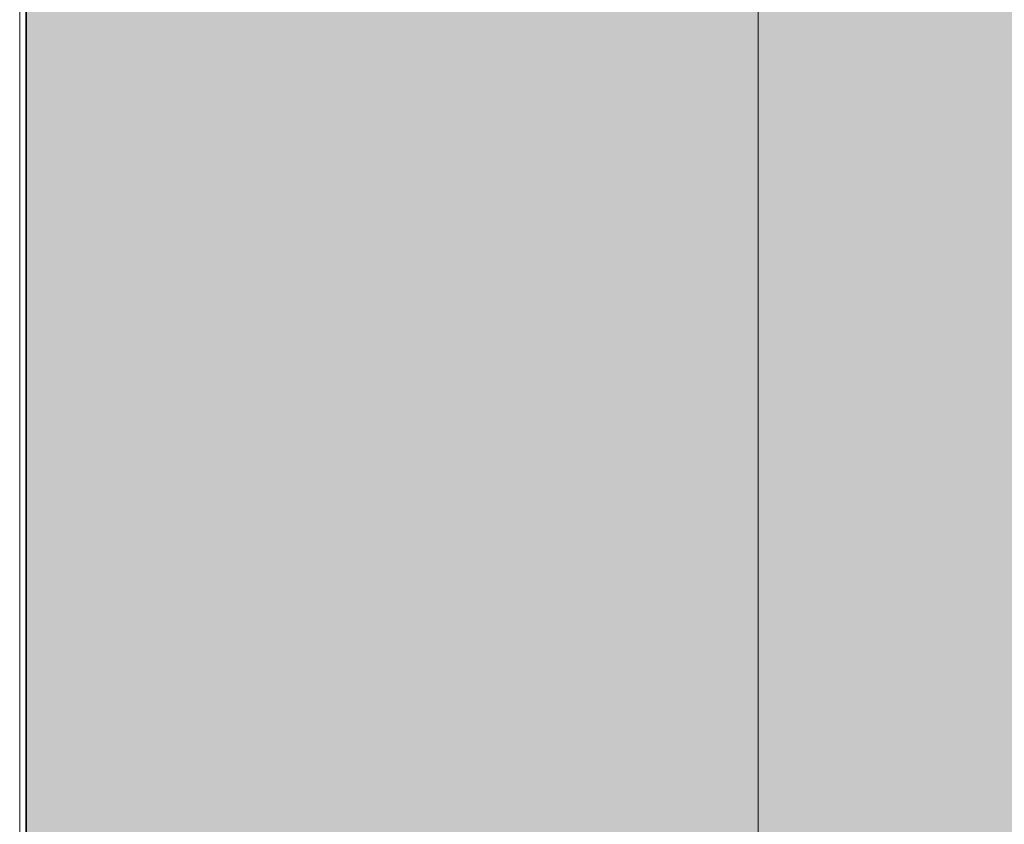
# Model space of a CAD drawing. Units: inches. Extents: x 2091 to 2899, y 967 to 2217.
# Tile 237 of 256: x 2203.116 to 2207.329, y 1155.69 to 1159.133. Entities that reach past the tile are written whole.
import ezdxf

# ---------------------------------------------------------------- set-up
doc = ezdxf.new("R2010")
doc.units = ezdxf.units.IN
doc.layers.add('A-GLAZ', color=4, linetype='Continuous', lineweight=18)
doc.layers.add('C-PROP', color=7, linetype='Continuous', lineweight=35)
doc.layers.add('A-WALL-PATT', color=141, linetype='Continuous', lineweight=13, true_color=0xadddf7)

# ---------------------------------------------------------------- blocks, each defined once
blk = doc.blocks.new('WIN-DOUBLE-LINE')
for p, q in [((0.0004, -0.0004), (0.0004, 80.8229)), ((3.1603, 80.8229), (3.1603, -0.0004))]:
    blk.add_line(p, q)

msp = doc.modelspace()

# ---------------------------------------------------------------- hatches: boundary and pattern name
at = {"layer": 'A-WALL-PATT'}
h = msp.add_hatch(color=256, dxfattribs=at)
h.dxf.hatch_style = 1
h.paths.add_polyline_path([(2803.1436, 2050.9191), (2203.1436, 2050.9191), (2203.1436, 1090.9191), (2803.1436, 1090.9191)])
h.paths.add_polyline_path([(2635.7989, 1147.5405), (2674.5241, 1147.5405, 0.376086), (2678.5297, 1152.8802), (2678.5297, 1159.5565, 0.333335), (2674.5243, 1163.5618), (2674.5243, 1163.5619), (2674.5243, 1192.9344), (2635.806, 1192.9344), (2597.0876, 1192.9344), (2597.0876, 1163.5618, 0.333335), (2593.0823, 1159.5565), (2593.0823, 1152.8802, 0.376086), (2597.0879, 1147.5405)], flags=0)
h.paths.add_polyline_path([(2436.0104, 1278.2408, 0.000483), (2435.9526, 1278.215, -0.001328), (2435.9356, 1278.1117, -0.001711), (2436.1164, 1278.0408, 0.002185)], flags=0)
h.paths.add_polyline_path([(2794.1436, 1143.4191), (2794.1436, 1347.4191), (2543.3702, 1347.4191), (2543.3702, 1351.9191), (2794.1436, 1351.9191), (2794.1436, 1392.7136), (2793.9474, 1392.7136), (2793.9474, 1473.5369), (2794.1436, 1473.5369), (2794.1436, 1531.9191), (2650.1436, 1531.9191), (2650.1436, 1536.4191), (2794.1436, 1536.4191), (2794.1436, 1692.4191), (2609.3756, 1692.4191), (2609.3756, 1644.4191), (2604.8756, 1644.4191), (2604.8756, 1744.9191), (2609.3756, 1744.9191), (2609.3756, 1696.9191), (2794.1436, 1696.9191), (2794.1436, 1780.9191), (2609.6436, 1780.9191), (2493.8756, 1780.9191), (2493.8756, 1785.4191), (2609.6436, 1785.4191), (2794.1436, 1785.4191), (2794.1436, 1847.9388), (2793.9512, 1847.9388), (2793.9512, 1928.7622), (2794.1436, 1928.7622), (2794.1436, 1941.4191), (2614.1436, 1941.4191), (2614.1436, 1821.4191), (2609.6436, 1821.4191), (2609.6436, 1941.4191), (2392.1436, 1941.4191), (2392.1436, 1819.9191), (2387.6436, 1819.9191), (2387.6436, 1941.4191), (2212.1436, 1941.4191), (2212.1436, 1783.9191), (2392.1436, 1783.9191), (2392.1436, 1780.9191), (2212.1436, 1780.9191), (2212.1436, 1629.4191), (2387.6436, 1629.4191), (2387.6436, 1744.9191), (2392.1436, 1744.9191), (2392.1436, 1627.9191), (2317.1436, 1627.9191), (2317.1436, 1551.4191), (2317.1436, 1536.4191), (2459.3836, 1536.4191), (2459.3836, 1602.3965), (2463.8836, 1602.3965), (2463.8836, 1531.9191), (2456.6436, 1531.9191), (2456.6436, 1529.9191), (2452.1436, 1529.9191), (2452.1436, 1531.9191), (2312.6436, 1531.9191), (2312.6436, 1551.4191), (2306.1436, 1551.4191), (2306.1436, 1555.9191), (2308.1436, 1555.9191), (2308.1436, 1551.4191), (2312.6436, 1551.4191), (2312.6436, 1627.9191), (2212.1436, 1627.9191), (2212.1436, 1555.9191), (2270.1436, 1555.9191), (2270.1436, 1551.4191), (2212.1436, 1551.4191), (2212.1436, 1351.9191), (2272.1436, 1351.9191), (2272.1436, 1347.4191), (2212.1436, 1347.4191), (2212.1436, 1275.4191), (2308.1436, 1275.4191), (2308.1436, 1351.9191), (2452.1436, 1351.9191), (2452.1436, 1493.9191), (2456.6436, 1493.9191), (2456.6436, 1347.4191), (2312.6436, 1347.4191), (2312.6436, 1270.9191), (2212.1436, 1270.9191), (2212.1436, 1099.9191), (2281.2375, 1099.9191), (2282.871, 1110.9138), (2282.0083, 1116.9966), (2278.5577, 1121.4204), (2268.2056, 1128.0562), (2272.0876, 1128.0562), (2273.8129, 1131.927), (2279.4203, 1134.6919), (2285.0278, 1135.2449), (2287.6158, 1137.4568), (2288.0471, 1138.0098), (2289.3411, 1140.7747), (2291.0665, 1139.6687), (2292.3605, 1135.2449), (2295.3798, 1136.9038), (2296.2425, 1135.7979), (2297.1052, 1133.033), (2300.1246, 1138.0098), (2303.1439, 1138.0098), (2304.4379, 1135.7979), (2303.1439, 1133.586), (2306.5946, 1134.6919), (2307.8887, 1133.033), (2310.908, 1135.2449), (2313.9274, 1134.1389), (2315.6269, 1132.4271), (2308.32, 1117.5496), (2290.2038, 1109.8079), (2288.9098, 1103.1721), (2289.2723, 1099.9191), (2434.9182, 1099.9191), (2431.5932, 1124.7881), (2429.9302, 1169.5531), (2430.9272, 1240.5197), (2435.6589, 1238.1861), (2437.1352, 1196.5541), (2438.7982, 1143.9731), (2442.6782, 1111.9981), (2446.5582, 1099.9191), (2794.1436, 1099.9191), (2794.1436, 1138.9191), (2548.0324, 1138.9191), (2548.0324, 1143.4191), (2548.0324, 1148.8191), (2546.6685, 1148.0316), (2528.6857, 1179.1786, 0.256256), (2512.0324, 1148.8191), (2512.0324, 1143.4191), (2512.0324, 1138.9191), (2507.5324, 1138.9191), (2507.5324, 1143.4191), (2507.5324, 1148.8191, 0.256256), (2490.8792, 1179.1786), (2472.8964, 1148.0316), (2471.5324, 1148.8191), (2471.5324, 1143.4191), (2467.0324, 1143.4191), (2467.0324, 1269.9458, 0.039061), (2460.91, 1273.5801), (2467.0324, 1273.5801), (2467.0324, 1286.3254, 0.014511), (2465.2162, 1286.7619), (2467.0324, 1287.0526), (2467.0324, 1323.4191), (2471.5324, 1323.4191), (2471.5324, 1148.8191), (2489.5324, 1179.996), (2490.8964, 1179.2085), (2490.8792, 1179.1786, -0.256256), (2507.5324, 1148.8191), (2507.5324, 1143.4191), (2512.0324, 1143.4191), (2512.0324, 1148.8191, -0.256256), (2528.6857, 1179.1786), (2528.6685, 1179.2085), (2530.0324, 1179.996), (2548.0324, 1148.8191), (2548.0324, 1143.4191)], flags=16)
h.paths.add_polyline_path([(2607.7685, 1200.9451), (2607.7685, 1265.0306), (2597.0876, 1281.052), (2619.7846, 1281.052), (2627.7953, 1337.1269), (2635.7989, 1337.1269), (2643.8167, 1337.1269), (2651.8274, 1281.052), (2674.5243, 1281.052), (2663.8434, 1265.0306), (2663.8434, 1200.9451), (2635.806, 1200.9451)], flags=0)
edge = h.paths.add_edge_path(flags=0)
edge.add_ellipse((13303.8962, 1272.9987), major_axis=(-10595.313, 0), ratio=0.8423038701, start_angle=0.62823722, end_angle=0.6465541, ccw=False)
edge.add_ellipse((2711.7004, 1156.8527), major_axis=(2.2198, 0), ratio=0.842304, start_angle=111.5352, end_angle=180.6282, ccw=False)
edge.add_ellipse((13303.1563, 1272.9987), major_axis=(-10593.0263, 0), ratio=0.8423038695, start_angle=0.52827147, end_angle=0.6465541, ccw=False)
edge.add_line((2710.7646, 1175.3333), (2710.13, 1175.3333))
edge.add_ellipse((2710.13, 1176.5798), major_axis=(1.4798, 0), ratio=0.842304, start_angle=180, end_angle=270, ccw=False)
edge.add_line((2708.6501, 1176.5798), (2708.6501, 1200.7829))
edge.add_ellipse((2710.13, 1200.7829), major_axis=(1.4798, 0), ratio=0.842304, start_angle=90, end_angle=180, ccw=False)
edge.add_line((2710.13, 1202.0294), (2710.4651, 1202.0294))
edge.add_ellipse((13303.1563, 1272.9987), major_axis=(-10593.0263, 0), ratio=0.8423038695, start_angle=-0.09022909, end_angle=0.38386678, ccw=False)
edge.add_ellipse((2710.13, 1290.927), major_axis=(-1.4798, 0), ratio=0.842304, start_angle=0, end_angle=90, ccw=False)
edge.add_line((2708.6501, 1290.927), (2708.6501, 1315.1302))
edge.add_ellipse((2710.13, 1315.1302), major_axis=(-1.4798, 0), ratio=0.842304, start_angle=-90, end_angle=0, ccw=False)
edge.add_line((2710.13, 1316.3767), (2710.7063, 1316.3767))
edge.add_ellipse((3238.4017, 1296.2896), major_axis=(528.234, 0), ratio=0.84230387, start_angle=176.349572, end_angle=177.82005, ccw=False)
edge.add_ellipse((2775.063, 1071.4507), major_axis=(313.3078, 0), ratio=0.84230387, start_angle=102.125966, end_angle=103.780529, ccw=False)
edge.add_ellipse((2775.063, 1078.3057), major_axis=(-305.3029, 0), ratio=0.84230387, start_angle=-79.790461, end_angle=-77.555373, ccw=False)
edge.add_ellipse((2695.1418, 1541.9754), major_axis=(-250.9602, 0), ratio=0.84230387, start_angle=99.256566, end_angle=102.554933)
edge.add_line((2741.4103, 1334.2143), (2747.1325, 1337.3785))
edge.add_ellipse((2747.5386, 1336.8575), major_axis=(-0.7399, 0), ratio=0.842304, start_angle=270, end_angle=307.9331, ccw=False)
edge.add_ellipse((2747.5386, 1336.8575), major_axis=(-0.7399, 0), ratio=0.842304, start_angle=232.0669, end_angle=270, ccw=False)
edge.add_line((2747.9447, 1337.3785), (2753.6669, 1334.2143))
edge.add_ellipse((2799.9355, 1541.9754), major_axis=(250.9602, 0), ratio=0.84230387, start_angle=257.445067, end_angle=260.743434)
edge.add_ellipse((2720.0142, 1078.3057), major_axis=(305.3029, 0), ratio=0.84230387, start_angle=77.555373, end_angle=79.790461, ccw=False)
edge.add_ellipse((2720.0142, 1071.4507), major_axis=(-313.3078, 0), ratio=0.84230387, start_angle=256.219471, end_angle=257.874034, ccw=False)
edge.add_ellipse((2256.6755, 1296.2896), major_axis=(-528.234, 0), ratio=0.84230387, start_angle=182.17995, end_angle=183.650428, ccw=False)
edge.add_line((2784.3709, 1316.3767), (2784.9472, 1316.3767))
edge.add_ellipse((2784.9472, 1315.1302), major_axis=(1.4798, 0), ratio=0.842304, start_angle=0, end_angle=90, ccw=False)
edge.add_line((2786.4271, 1315.1302), (2786.4271, 1290.927))
edge.add_ellipse((2784.9472, 1290.927), major_axis=(1.4798, 0), ratio=0.842304, start_angle=270, end_angle=360, ccw=False)
edge.add_ellipse((-7808.0791, 1272.9987), major_axis=(10593.0263, 0), ratio=0.8423038695, start_angle=-0.38386678, end_angle=0.09022909, ccw=False)
edge.add_line((2784.6122, 1202.0294), (2784.9472, 1202.0294))
edge.add_ellipse((2784.9472, 1200.7829), major_axis=(1.4798, 0), ratio=0.842304, start_angle=0, end_angle=90, ccw=False)
edge.add_line((2786.4271, 1200.7829), (2786.4271, 1176.5798))
edge.add_ellipse((2784.9472, 1176.5798), major_axis=(-1.4798, 0), ratio=0.842304, start_angle=90, end_angle=180, ccw=False)
edge.add_line((2784.9472, 1175.3333), (2784.3126, 1175.3333))
edge.add_ellipse((-7808.0791, 1272.9987), major_axis=(10593.0263, 0), ratio=0.8423038695, start_angle=-0.6186432, end_angle=-0.52827147, ccw=False)
edge.add_ellipse((2783.3768, 1156.8527), major_axis=(-2.2198, 0), ratio=0.842304, start_angle=179.3718, end_angle=248.4648, ccw=False)
edge.add_ellipse((-7808.819, 1272.9987), major_axis=(-10595.313, 0), ratio=0.8423038658, start_angle=179.35344592, end_angle=179.3717628, ccw=False)
edge.add_ellipse((2780.2973, 1153.5008), major_axis=(-5.2464, 0), ratio=0.842304, start_angle=90, end_angle=179.3534, ccw=False)
edge.add_line((2780.2973, 1149.0817), (2714.7799, 1149.0817))
edge.add_ellipse((2714.7799, 1153.5008), major_axis=(5.2464, 0), ratio=0.842304, start_angle=180.6466, end_angle=270, ccw=False)
edge = h.paths.add_edge_path(flags=0)
edge.add_line((2718.1874, 1151.0078), (2718.1874, 1170.4724))
edge.add_ellipse((2721.1471, 1170.4724), major_axis=(-2.9597, 0), ratio=0.842304, start_angle=-90, end_angle=0, ccw=False)
edge.add_line((2721.1471, 1172.9653), (2773.9302, 1172.9653))
edge.add_ellipse((2773.9302, 1170.4724), major_axis=(-2.9597, 0), ratio=0.842304, start_angle=180, end_angle=270, ccw=False)
edge.add_line((2776.8899, 1170.4724), (2776.8899, 1151.0078))
edge.add_line((2776.8899, 1151.0078), (2718.1874, 1151.0078))
edge = h.paths.add_edge_path(flags=0)
edge.add_line((2718.1874, 1180.2342), (2718.1874, 1199.0578))
edge.add_ellipse((2747.5386, 1320.3986), major_axis=(147.0179, 0), ratio=0.84230387, start_angle=256.401865, end_angle=283.598135)
edge.add_line((2776.8899, 1199.0578), (2776.8899, 1180.2342))
edge.add_ellipse((2747.5386, 1301.575), major_axis=(147.0179, 0), ratio=0.84230387, start_angle=256.401865, end_angle=283.598135, ccw=False)
edge = h.paths.add_edge_path(flags=0)
edge.add_ellipse((13303.1563, 1272.9987), major_axis=(-10591.5465, 0), ratio=0.8423038696, start_angle=0.05559431, end_angle=0.37776419, ccw=False)
edge.add_line((2711.6169, 1262.7217), (2715.6674, 1249.4954))
edge.add_ellipse((6413.892, 1241.6919), major_axis=(-3698.2362, 0), ratio=0.84230387, start_angle=-0.1208974, end_angle=0.3640763)
edge.add_line((2715.761, 1218.1925), (2711.9343, 1203.1674))
edge = h.paths.add_edge_path(flags=0)
edge.add_line((2718.1874, 1251.0746), (2716.0025, 1267.4504))
edge.add_ellipse((2742.1512, 1202.1895), major_axis=(81.7726, 0), ratio=0.8423039, start_angle=94.277421, end_angle=111.834954, ccw=False)
edge.add_line((2737.0097, 1270.9306), (2758.0675, 1270.9306))
edge.add_ellipse((2752.9261, 1202.1895), major_axis=(81.7726, 0), ratio=0.8423039, start_angle=68.165046, end_angle=85.722579, ccw=False)
edge.add_line((2779.0747, 1267.4504), (2776.8899, 1251.0746))
edge.add_ellipse((2750.3381, 1187.8854), major_axis=(79.5797, 0), ratio=0.8423039, start_angle=67.208085, end_angle=85.12993)
edge.add_line((2756.0347, 1254.7437), (2739.0426, 1254.7437))
edge.add_ellipse((2744.7392, 1187.8854), major_axis=(79.5797, 0), ratio=0.8423039, start_angle=94.87007, end_angle=112.791915)
edge = h.paths.add_edge_path(flags=0)
edge.add_line((2783.1429, 1203.1674), (2779.3162, 1218.1925))
edge.add_ellipse((-918.8147, 1241.6919), major_axis=(3698.2362, 0), ratio=0.84230387, start_angle=-0.3640763, end_angle=0.1208974)
edge.add_line((2779.4098, 1249.4954), (2783.4604, 1262.7217))
edge.add_ellipse((-7808.0791, 1272.9987), major_axis=(-10591.5465, 0), ratio=0.8423038695, start_angle=179.62223581, end_angle=179.94440569, ccw=False)
edge = h.paths.add_edge_path(flags=0)
edge.add_ellipse((2734.2009, 1286.6904), major_axis=(-0.3566, 6.3401), ratio=0.603834, start_angle=89.00201, end_angle=253.65741, ccw=False)
edge.add_line((2730.369, 1286.5418), (2730.369, 1301.352))
edge.add_line((2730.369, 1301.352), (2735.9133, 1305.2148))
edge.add_ellipse((2736.3849, 1304.7346), major_axis=(0.7399, 0), ratio=0.842304, start_angle=90, end_angle=134.4802, ccw=False)
edge.add_line((2736.3849, 1305.3578), (2738.0328, 1305.3578))
edge.add_line((2738.0328, 1305.3578), (2738.0328, 1307.7079))
edge.add_ellipse((2794.2016, 1307.7079), major_axis=(56.1689, 0), ratio=0.8423039, start_angle=150.56143, end_angle=180, ccw=False)
edge.add_ellipse((2700.8756, 1307.7079), major_axis=(-56.1689, 0), ratio=0.8423039, start_angle=180, end_angle=209.43857, ccw=False)
edge.add_line((2757.0444, 1307.7079), (2757.0444, 1305.3578))
edge.add_line((2757.0444, 1305.3578), (2758.6923, 1305.3578))
edge.add_ellipse((2758.6923, 1304.7346), major_axis=(-0.7399, 0), ratio=0.842304, start_angle=225.5198, end_angle=270, ccw=False)
edge.add_line((2759.1639, 1305.2148), (2764.7082, 1301.352))
edge.add_line((2764.7082, 1301.352), (2764.7082, 1286.5418))
edge.add_ellipse((2760.8763, 1286.6904), major_axis=(0.3566, 6.3401), ratio=0.603834, start_angle=106.34259, end_angle=270.99799, ccw=False)
edge.add_line((2757.0444, 1285.7971), (2757.0444, 1307.7079))
edge.add_ellipse((2700.8756, 1307.7079), major_axis=(-56.1689, 0), ratio=0.8423039, start_angle=180, end_angle=209.43857)
edge.add_ellipse((2794.2016, 1307.7079), major_axis=(56.1689, 0), ratio=0.8423039, start_angle=150.56143, end_angle=180)
edge.add_line((2738.0328, 1307.7079), (2738.0328, 1285.7971))
h.paths.add_polyline_path([(2417.8123, 1104.4497), (2413.4923, 1102.5297), (2410.6123, 1103.9697), (2409.1723, 1106.3697), (2407.2523, 1107.3297), (2406.2923, 1109.7297), (2405.3323, 1114.0497), (2405.3323, 1117.8897), (2406.2923, 1120.1297), (2407.2523, 1119.8097), (2408.8483, 1118.3277), (2410.1739, 1119.4242), (2410.2113, 1120.4057), (2411.0407, 1121.4191), (2410.6993, 1119.8587), (2410.1739, 1119.4242), (2410.0885, 1117.1761), (2411.1328, 1116.2063), (2413.9723, 1119.3297), (2416.8523, 1120.7697), (2416.8697, 1120.7988), (2417.0351, 1119.4051), (2417.8962, 1118.1434), (2418.2923, 1118.3697), (2419.5444, 1120.0393), (2419.3609, 1118.3875), (2419.0321, 1119.3562), (2418.3989, 1118.5119), (2419.2523, 1114.5297), (2418.7941, 1107.1988)], flags=0)
h.paths.add_polyline_path([(2508.8702, 1347.4191), (2508.3702, 1347.4191), (2508.3702, 1351.9191), (2508.8702, 1351.9191)], flags=0)
h.paths.add_polyline_path([(2473.3702, 1347.4191), (2472.3702, 1347.4191), (2467.8702, 1347.4191), (2467.8702, 1455.4191), (2472.3702, 1455.4191), (2472.3702, 1352.4191), (2473.3702, 1352.4191)], flags=0)
h.paths.add_polyline_path([(2352.1062, 1217.4462), (2349.2262, 1218.8862), (2347.7862, 1221.2862), (2345.8662, 1222.2462), (2344.9062, 1224.6462), (2343.9462, 1228.9662), (2343.9462, 1232.8062), (2344.9062, 1235.0462), (2345.8662, 1234.7262), (2347.4623, 1233.2442), (2348.7879, 1234.3407), (2348.8252, 1235.3222), (2349.6547, 1236.3355), (2349.3132, 1234.7752), (2348.7879, 1234.3407), (2348.7024, 1232.0926), (2349.7468, 1231.1228), (2352.5862, 1234.2462), (2355.4662, 1235.6862), (2355.4837, 1235.7153), (2355.649, 1234.3216), (2356.5102, 1233.0599), (2356.9062, 1233.2862), (2358.1584, 1234.9558), (2357.9749, 1233.304), (2357.6461, 1234.2726), (2357.0129, 1233.4284), (2357.8662, 1229.4462), (2357.4081, 1222.1153), (2356.4262, 1219.3662)], flags=0)
h.paths.add_polyline_path([(2348.2968, 1112.2244), (2347.0138, 1112.3104), (2345.5298, 1114.1274), (2345.7318, 1115.8584), (2346.8118, 1116.9824), (2346.8118, 1114.6464), (2345.8668, 1114.2144), (2346.8798, 1114.3004)], flags=0)
h.paths.add_polyline_path([(2347.0138, 1110.9264), (2346.2718, 1110.4934), (2346.6098, 1111.1864)], flags=0)
h.paths.add_polyline_path([(2345.8668, 1118.1944), (2345.5298, 1117.3294), (2343.7078, 1118.0214), (2344.3828, 1118.6264)], flags=0)
h.paths.add_polyline_path([(2346.6768, 1109.2824), (2346.0698, 1108.0714), (2345.8668, 1110.0614)], flags=0)
h.paths.add_polyline_path([(2345.0568, 1119.7514), (2343.6398, 1119.7514), (2343.9778, 1121.1354)], flags=0)
h.paths.add_polyline_path([(2345.2598, 1116.5504), (2345.1248, 1115.8584), (2344.9218, 1115.6854), (2344.7198, 1116.3774)], flags=0)
h.paths.add_polyline_path([(2345.6648, 1112.3104), (2345.4618, 1111.5324), (2344.0448, 1111.9644), (2344.6518, 1112.5704)], flags=0)
h.paths.add_polyline_path([(2345.1918, 1113.3494), (2344.4498, 1113.8684), (2344.7198, 1114.3874)], flags=0)
h.paths.add_polyline_path([(2344.6518, 1116.8094), (2344.1798, 1115.6854), (2344.6518, 1115.3394), (2343.9098, 1114.9064), (2343.0328, 1115.9444), (2343.6398, 1116.4634)], flags=0)
h.paths.add_polyline_path([(2345.8668, 1106.6864), (2344.9898, 1105.5624), (2344.5168, 1106.6004)], flags=0)
h.paths.add_polyline_path([(2344.8548, 1110.0614), (2344.5168, 1109.2824), (2344.1128, 1109.7154)], flags=0)
h.paths.add_polyline_path([(2344.0448, 1113.5224), (2343.4378, 1113.0894), (2342.7628, 1113.9544)], flags=0)
h.paths.add_polyline_path([(2344.3148, 1111.0124), (2342.9648, 1110.3204), (2342.9648, 1111.0994)], flags=0)
h.paths.add_polyline_path([(2345.1248, 1104.6974), (2344.5848, 1103.7454), (2344.4498, 1104.2644)], flags=0)
h.paths.add_polyline_path([(2342.8298, 1121.2224), (2341.7498, 1120.5304), (2340.5358, 1121.0494), (2340.1308, 1121.8284), (2340.6708, 1122.9524), (2341.1428, 1121.8284), (2341.6148, 1122.0014)], flags=0)
h.paths.add_polyline_path([(2342.9648, 1119.7514), (2343.0328, 1118.4534), (2342.0878, 1118.0214), (2342.0198, 1119.4914)], flags=0)
h.paths.add_polyline_path([(2342.6948, 1116.8964), (2341.9528, 1116.6364), (2342.0198, 1117.3294)], flags=0)
h.paths.add_polyline_path([(2343.0328, 1112.2244), (2342.0198, 1111.7914), (2341.5478, 1112.2244), (2342.3578, 1113.3494)], flags=0)
h.paths.add_polyline_path([(2343.7748, 1104.4374), (2342.6278, 1102.8804), (2342.6948, 1104.6104), (2343.4378, 1105.1294)], flags=0)
h.paths.add_polyline_path([(2342.0198, 1115.0794), (2340.8058, 1115.5124), (2340.9408, 1116.3774)], flags=0)
h.paths.add_polyline_path([(2341.4808, 1120.0974), (2341.4808, 1119.4054), (2341.0758, 1119.5784), (2341.1428, 1120.0974)], flags=0)
h.paths.add_polyline_path([(2341.8178, 1114.4734), (2340.9408, 1113.0894), (2340.8058, 1114.5604)], flags=0)
h.paths.add_polyline_path([(2341.1428, 1118.5404), (2340.9408, 1116.9824), (2339.0508, 1117.6754), (2339.0508, 1118.6264)], flags=0)
h.paths.add_polyline_path([(2342.6948, 1101.6684), (2341.9528, 1101.8414), (2342.5598, 1102.3614)], flags=0)
h.paths.add_polyline_path([(2340.3328, 1119.6654), (2338.4438, 1119.5784), (2337.9038, 1120.3574), (2339.6578, 1120.6164)], flags=0)
h.paths.add_polyline_path([(2340.3328, 1115.3394), (2340.0628, 1113.6954), (2339.3878, 1115.3394)], flags=0)
h.paths.add_polyline_path([(2341.8178, 1103.8314), (2341.5478, 1102.8804), (2341.1428, 1103.6584)], flags=0)
h.paths.add_polyline_path([(2339.0508, 1122.8664), (2337.2958, 1121.8284), (2337.0938, 1123.1254), (2337.7688, 1123.8184)], flags=0)
h.paths.add_polyline_path([(2339.1178, 1121.7414), (2338.8478, 1121.2224), (2338.1738, 1121.0494), (2338.3758, 1121.5684)], flags=0)
h.paths.add_polyline_path([(2339.1858, 1119.3194), (2338.6458, 1118.7134), (2338.2408, 1118.1074), (2338.2408, 1118.8864)], flags=0)
h.paths.add_polyline_path([(2341.1428, 1101.9284), (2340.6028, 1101.2364), (2340.0628, 1101.8414), (2340.6028, 1102.3614)], flags=0)
h.paths.add_polyline_path([(2337.6338, 1117.7614), (2336.6208, 1118.2804), (2337.2958, 1118.9724)], flags=0)
h.paths.add_polyline_path([(2336.8238, 1119.5784), (2334.7988, 1118.9724), (2335.2038, 1120.3574), (2336.5538, 1120.8764)], flags=0)
h.paths.add_polyline_path([(2339.1178, 1100.4574), (2337.3638, 1100.5434), (2336.7558, 1101.2364)], flags=0)
h.paths.add_polyline_path([(2336.3508, 1122.4334), (2336.0138, 1121.9144), (2334.9338, 1122.4334), (2334.5288, 1123.4714), (2335.7438, 1122.7794)], flags=0)
h.paths.add_polyline_path([(2334.7318, 1120.8764), (2334.2588, 1120.3574), (2334.0568, 1120.7894), (2334.5968, 1121.3084)], flags=0)
h.paths.add_polyline_path([(2334.4618, 1122.1744), (2332.5718, 1121.3084), (2331.3568, 1122.1744), (2332.0998, 1122.8664)], flags=0)
h.paths.add_polyline_path([(2334.2588, 1118.5404), (2333.3818, 1118.4534), (2333.6518, 1119.3194)], flags=0)
h.paths.add_polyline_path([(2335.5418, 1102.2744), (2334.1918, 1102.6204), (2335.2718, 1103.3124)], flags=0)
h.paths.add_polyline_path([(2332.7068, 1119.6654), (2331.6948, 1120.4434), (2332.5048, 1120.7894)], flags=0)
h.paths.add_polyline_path([(2334.7318, 1101.1494), (2333.5168, 1101.5824), (2333.9888, 1101.7554)], flags=0)
h.paths.add_polyline_path([(2332.6398, 1116.6364), (2331.0868, 1116.2904), (2331.9648, 1118.1944)], flags=0)
h.paths.add_polyline_path([(2330.7498, 1121.5684), (2330.2768, 1120.2704), (2328.5228, 1119.3194), (2328.9948, 1121.0494)], flags=0)
h.paths.add_polyline_path([(2330.7498, 1118.6264), (2330.0078, 1117.5024), (2329.8728, 1118.0214)], flags=0)
h.paths.add_polyline_path([(2332.0998, 1102.3614), (2330.5468, 1102.0144), (2331.6948, 1102.9664)], flags=0)
h.paths.add_polyline_path([(2329.5348, 1113.6084), (2329.0628, 1112.3104), (2328.5898, 1113.3494)], flags=0)
h.paths.add_polyline_path([(2328.3878, 1117.8484), (2327.5098, 1116.5504), (2327.1728, 1117.7614)], flags=0)
h.paths.add_polyline_path([(2329.7378, 1106.5134), (2329.5348, 1105.3024), (2328.2528, 1106.0814)], flags=0)
h.paths.add_polyline_path([(2328.6578, 1114.3874), (2328.0498, 1114.1274), (2328.3198, 1114.9064)], flags=0)
h.paths.add_polyline_path([(2328.3198, 1112.2244), (2327.1058, 1112.1374), (2326.7008, 1112.6564)], flags=0)
h.paths.add_polyline_path([(2326.9028, 1115.2524), (2326.7008, 1114.1274), (2325.2158, 1113.6084), (2326.0928, 1115.3394)], flags=0)
h.paths.add_polyline_path([(2326.6328, 1108.3304), (2326.0928, 1107.3794), (2325.8908, 1108.5034), (2326.4978, 1109.1094)], flags=0)
h.paths.add_polyline_path([(2615.1436, 1531.9191), (2609.6436, 1531.9191), (2609.6436, 1620.4191), (2614.1436, 1620.4191), (2614.1436, 1536.4191), (2615.1436, 1536.4191)], flags=0)
h.paths.add_polyline_path([(2545.1436, 1563.4191), (2464.1436, 1563.4191), (2464.1436, 1632.4191), (2509.1436, 1632.4191), (2509.1436, 1627.9191), (2509.1436, 1603.9191), (2468.6436, 1603.9191), (2468.6436, 1567.9191), (2540.6436, 1567.9191), (2540.6436, 1591.9191), (2545.1436, 1591.9191)], flags=0)
h.paths.add_polyline_path([(2388.969, 1549.9857), (2357.4342, 1549.9857), (2357.4342, 1623.3608), (2399.3628, 1623.3608), (2435.6895, 1623.3608), (2435.5925, 1602.5593), (2435.5925, 1602.3965), (2388.969, 1602.3965)], flags=0)
h.paths.add_polyline_path([(2388.8806, 1555.8092), (2374.9044, 1555.8092), (2374.9044, 1600.5716), (2374.9044, 1615.4576), (2406.3509, 1615.4576), (2406.3509, 1618.9394), (2412.1743, 1615.4576), (2406.3509, 1611.9759), (2406.3509, 1615.4576), (2388.8806, 1615.4576)], flags=0)
h.paths.add_polyline_path([(2568.8756, 1644.4191), (2453.3756, 1644.4191), (2453.3756, 1785.4191), (2457.8756, 1785.4191), (2457.8756, 1648.9191), (2568.8756, 1648.9191)], flags=0)
h.paths.add_polyline_path([(2212.1436, 1945.9191), (2212.1436, 2041.9191), (2794.1436, 2041.9191), (2794.1436, 1945.9191)], flags=16)
h.paths.add_polyline_path([(2271.0827, 1964.3172), (2776.853, 1964.3172), (2776.853, 2037.1696), (2271.0827, 2037.1696)], flags=8)
h.paths.add_polyline_path([(2380.6493, 1536.8241), (2461.0408, 1536.8241), (2461.0408, 1554.6526), (2380.6493, 1554.6526)], flags=8)
h.paths.add_polyline_path([(2240.7557, 1609.7255), (2309.1858, 1609.7255), (2309.1858, 1617.6982), (2240.7557, 1617.6982)], flags=8)
h.paths.add_polyline_path([(2212.6773, 1313.5041), (2282.5915, 1313.5041), (2282.5915, 1322.7452), (2212.6773, 1322.7452)], flags=8)
h.paths.add_polyline_path([(2457.112, 1114.7786), (2558.4816, 1114.7786), (2558.4816, 1142.2197), (2457.112, 1142.2197)], flags=8)
h.paths.add_polyline_path([(2473.4423, 1273.0101), (2604.6412, 1273.0101), (2604.6412, 1318.3469), (2473.4423, 1318.3469)], flags=8)
h.paths.add_polyline_path([(2638.8763, 1626.9774), (2684.2504, 1627.9767), (2684.0385, 1637.5975), (2638.6644, 1636.5982)], flags=8)
h.paths.add_polyline_path([(2537.5906, 1453.7934), (2628.3895, 1453.7934), (2628.3895, 1475.3448), (2537.5906, 1475.3448)], flags=8)
h.paths.add_polyline_path([(2504.1376, 1714.6324), (2554.6472, 1714.6324), (2554.6472, 1730.2377), (2504.1376, 1730.2377)], flags=8)
h.paths.add_polyline_path([(2487.5012, 1575.6519), (2535.0971, 1575.6519), (2535.0971, 1598.3776), (2487.5012, 1598.3776)], flags=8)
h.paths.add_polyline_path([(2709.0994, 1735.7103), (2740.0166, 1735.7103), (2740.0166, 1749.9376), (2709.0994, 1749.9376)], flags=8)
h.paths.add_polyline_path([(2442.4384, 1792.1717), (2564.7288, 1792.1717), (2564.7288, 1842.0002), (2442.4384, 1842.0002)], flags=8)
h.paths.add_polyline_path([(2655.8158, 1809.6441), (2789.5201, 1806.6938), (2790.085, 1832.2916), (2656.3806, 1835.2419)], flags=8)
h.paths.add_polyline_path([(2234.8427, 1797.7201), (2368.5929, 1794.7689), (2369.1607, 1820.5041), (2235.4106, 1823.4554)], flags=8)
h.paths.add_polyline_path([(2245.1385, 1644.0063), (2398.4277, 1640.6239), (2398.9948, 1666.3248), (2245.7056, 1669.7073)], flags=8)
h.paths.add_polyline_path([(2306.1428, 1431.1685), (2413.7683, 1428.7937), (2414.3331, 1454.3915), (2306.7077, 1456.7664)], flags=8)
h.paths.add_polyline_path([(2306.8346, 1458.2331), (2393.3805, 1456.3234), (2393.9328, 1481.3544), (2307.3869, 1483.2641)], flags=8)

# ---------------------------------------------------------------- linework, layer by layer
at = {"layer": 'C-PROP'}
msp.add_lwpolyline([(2203.1436, 2050.9191), (2803.1436, 2050.9191), (2803.1436, 1090.9191), (2203.1436, 1090.9191)], close=True, dxfattribs=at)

# ---------------------------------------------------------------- block references
at = {"layer": 'A-GLAZ'}
msp.add_blockref('WIN-DOUBLE-LINE', (2203.1153, 1152.2475), dxfattribs=at)

doc.saveas('drawing.dxf')
